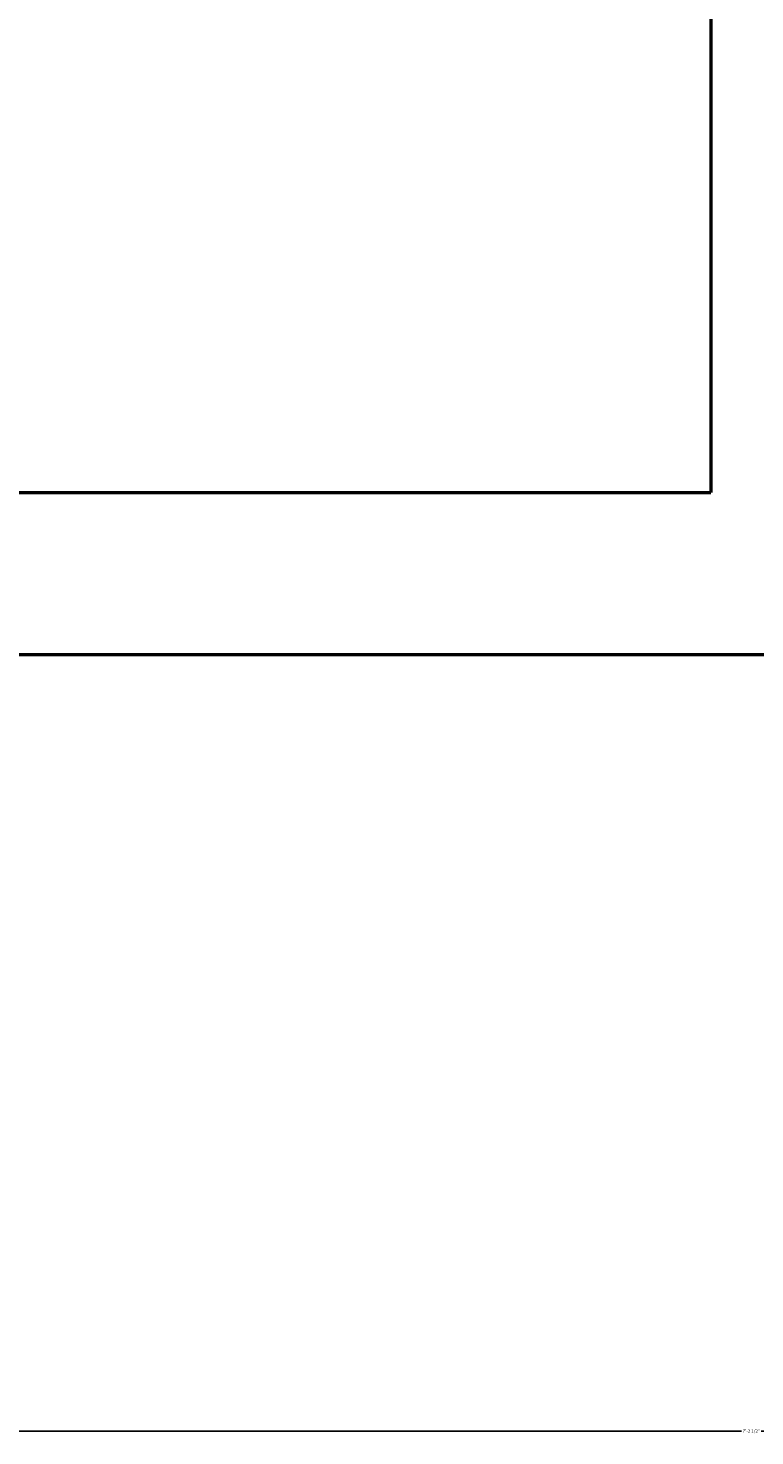
# Model space of a CAD drawing. Units: inches. Extents: x -173 to 545, y -746 to 104.
# Tile 6 of 32: x 223 to 263, y -741 to -663. Entities that reach past the tile are written whole.
import ezdxf

# ---------------------------------------------------------------- set-up
doc = ezdxf.new("R2010")
doc.units = ezdxf.units.IN
doc.header["$MEASUREMENT"] = 0
doc.layers.add('A-ANNO-DIMS', color=2, linetype='Continuous', lineweight=18)
doc.layers.add('A-WALL', color=7, linetype='Continuous', lineweight=50)
doc.styles.get("Standard").update_dxf_attribs({"font": 'arial.ttf'})
doc.dimstyles.get("Standard").update_dxf_attribs({"dimtxt": 0.18, "dimasz": 0.18, "dimexe": 0.18, "dimexo": 0.0625, "dimgap": 0.09, "dimtad": 0, "dimtih": 1, "dimtoh": 1, "dimdec": 0, "dimzin": 0, "dimdsep": 46, "dimlunit": 3, "dimtxsty": 'Standard', "dimcen": 0.09, "dimadec": 0, "dimazin": 0, "dimtfac": 1, "dimtdec": 0, "dimtofl": 0, "dimtmove": 0, "dimatfit": 3, "dimfxl": 1, "dimtolj": 1, "dimtzin": 0, "dimarcsym": 0})

# ---------------------------------------------------------------- blocks, each defined once
blk = doc.blocks.new('*D81')
at = {"layer": 'A-ANNO-DIMS', "color": 0, "lineweight": -2, "transparency": 16777216}
for p, q in [((219.801, -551.924), (219.801, -740.642)), ((306.301, -551.924), (306.301, -740.642)), ((219.981, -740.462), (262.513, -740.462)), ((306.121, -740.462), (263.59, -740.462))]:
    blk.add_line(p, q, dxfattribs=at)
at = {"layer": 'A-ANNO-DIMS', "color": 0, "transparency": 16777216}
for points in [[(219.981, -740.432), (219.981, -740.492), (219.801, -740.462)], [(306.121, -740.432), (306.121, -740.492), (306.301, -740.462)]]:
    blk.add_solid(points, dxfattribs=at)
at = {"layer": 'Defpoints', "color": 0, "transparency": 16777216}
for p in [(219.801, -551.862), (306.301, -551.862), (306.301, -740.462)]:
    blk.add_point(p, dxfattribs=at)
at = {"layer": 'A-ANNO-DIMS', "color": 0, "transparency": 16777216, "insert": (263.051, -740.462), "char_height": 0.18, "attachment_point": 5}
blk.add_mtext('\\A1;7\'-2 1/2"', dxfattribs=at)

msp = doc.modelspace()

# ---------------------------------------------------------------- linework, layer by layer
at = {"layer": 'A-WALL'}
for p, q in [((260.801, -560.862), (260.801, -688.362)), ((169.801, -688.362), (260.801, -688.362)), ((24.301, -697.362), (501.801, -697.362))]:
    msp.add_line(p, q, dxfattribs=at)

# ---------------------------------------------------------------- dimensions: what is measured, and where the dimension line sits
at = {"layer": 'A-ANNO-DIMS'}
dim = msp.add_linear_dim(base=(306.301, -740.462), p1=(219.801, -551.862), p2=(306.301, -551.862), dimstyle='Standard', override={"dimdec": 1, "dimlfac": 1, "dimrnd": 0, "dimzin": 1, "dimdsep": 46, "dimlunit": 4, "dimfrac": 2}, dxfattribs=at)
dim.commit()
dim.dimension.update_dxf_attribs({"geometry": '*D81', "text_midpoint": (263.051, -740.462)})

doc.saveas('drawing.dxf')
